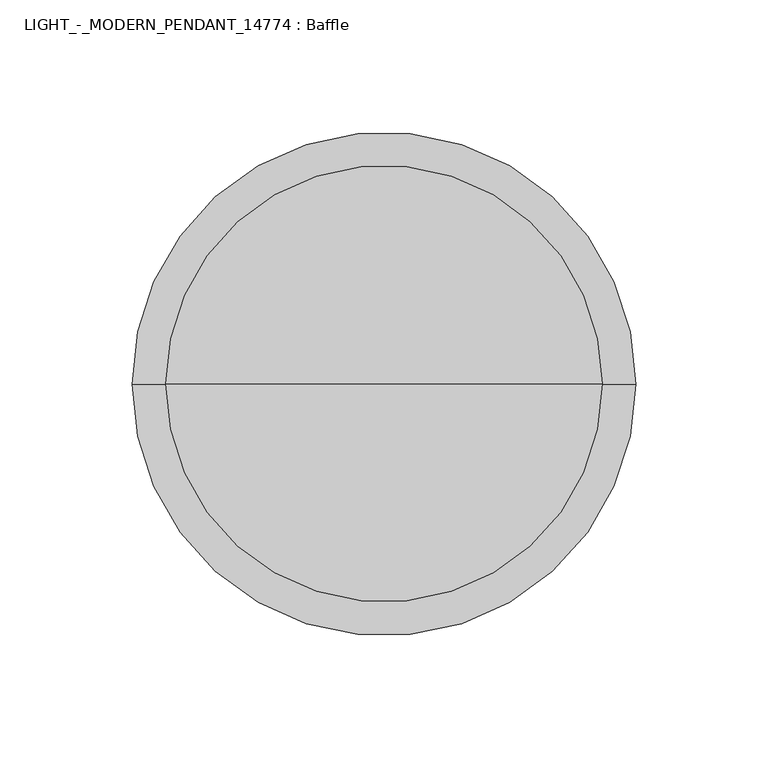
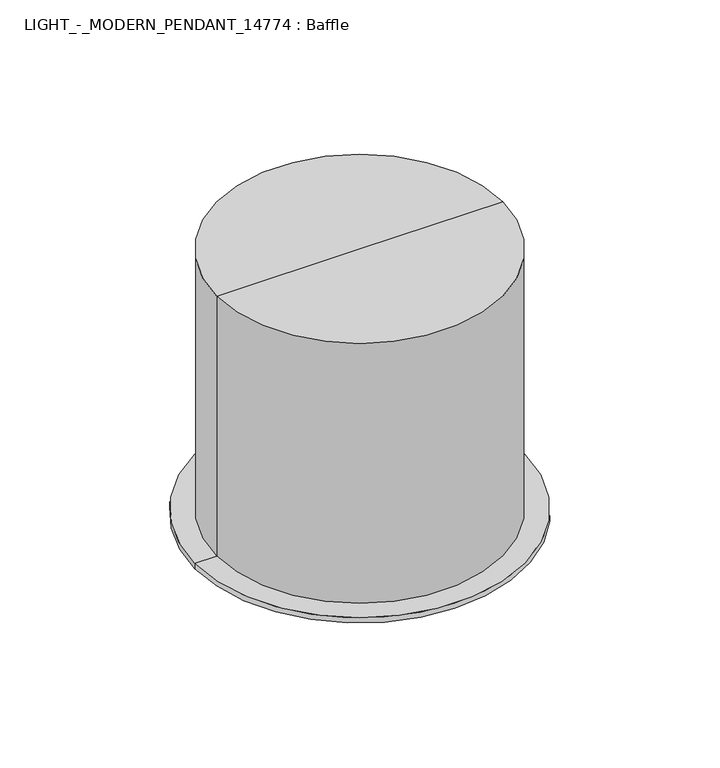
"""IFC4 building model written with IfcOpenShell, lengths in millimetres: light fixture geometry, LIGHT_-_MODERN_PENDANT_14774 : Baffle."""

from ifc_helpers import new_model, si_unit, frame, origin, place, context, project, spatial, polyline, circle_curve, source, transform, mapped, element, save
from ifc_brep_helpers import plane_surface, cylinder_surface, revolved_surface, advanced_brep


def light_modern_pendant_14774_baffle_cc9af11b(model_context):
    return source(origin(), model_context, "Body", "AdvancedBrep", [
        advanced_brep(
        [(-76.2, 0.0, 2438.4), (76.2, 0.0, 2438.4), (76.2, 0.0, 2590.8), (-76.2, 0.0, 2590.8), (-82.55, 0.0, 2438.4), (82.55, 0.0, 2438.4), (-82.55, 0.0, 2597.15), (82.55, 0.0, 2597.15), (0.0, 0.0, 2597.15), (0.0, 0.0, 2590.8)],
        [
            (0, 1, circle_curve(frame((0.0, 0.0, 2438.4), z_axis=(0.0, 0.0, -1.0), x_axis=(1.0, 0.0, 0.0)), 76.2)),
            (1, 2),
            (2, 3, circle_curve(frame((0.0, 0.0, 2590.8), z_axis=(0.0, 0.0, 1.0), x_axis=(1.0, 0.0, 0.0)), 76.2)),
            (3, 0),
            (1, 0, circle_curve(frame((0.0, 0.0, 2438.4), z_axis=(0.0, 0.0, -1.0), x_axis=(1.0, 0.0, 0.0)), 76.2)),
            (3, 2, circle_curve(frame((0.0, 0.0, 2590.8), z_axis=(0.0, 0.0, 1.0), x_axis=(1.0, 0.0, 0.0)), 76.2)),
            (4, 5, circle_curve(frame((0.0, 0.0, 2438.4), z_axis=(0.0, 0.0, -1.0), x_axis=(1.0, 0.0, 0.0)), 82.55)),
            (5, 1),
            (0, 4),
            (5, 4, circle_curve(frame((0.0, 0.0, 2438.4), z_axis=(0.0, 0.0, -1.0), x_axis=(1.0, 0.0, 0.0)), 82.55)),
            (6, 7, circle_curve(frame((0.0, 0.0, 2597.15), z_axis=(0.0, 0.0, -1.0), x_axis=(1.0, 0.0, 0.0)), 82.55)),
            (7, 5),
            (4, 6),
            (7, 6, circle_curve(frame((0.0, 0.0, 2597.15), z_axis=(0.0, 0.0, -1.0), x_axis=(1.0, 0.0, 0.0)), 82.55)),
            (8, 7),
            (6, 8),
            (2, 9),
            (9, 3),
        ],
        [
            revolved_surface(polyline([(76.2, 0.0, 2590.8), (76.2, 0.0, 2438.4)]), (0.0, 0.0, 2438.4), (0.0, 0.0, 1.0)),
            plane_surface(frame((0.0, 0.0, 2438.4), z_axis=(0.0, 0.0, -1.0), x_axis=(1.0, 0.0, 0.0))),
            cylinder_surface(frame((0.0, 0.0, 2438.4), z_axis=(0.0, 0.0, 1.0), x_axis=(1.0, 0.0, 0.0)), 82.55),
            plane_surface(frame((0.0, 0.0, 2597.15), z_axis=(0.0, 0.0, 1.0), x_axis=(1.0, 0.0, 0.0))),
            plane_surface(frame((0.0, 0.0, 2590.8), z_axis=(0.0, 0.0, -1.0), x_axis=(1.0, 0.0, 0.0))),
        ],
        [
            (0, [[1, 2, 3, 4]]),
            (0, [[5, -4, 6, -2]]),
            (1, [[7, 8, -1, 9]]),
            (1, [[10, -9, -5, -8]]),
            (2, [[11, 12, -7, 13]]),
            (2, [[14, -13, -10, -12]]),
            (3, [[15, -11, 16]]),
            (3, [[-16, -14, -15]]),
            (4, [[-3, 17, 18]]),
            (4, [[-6, -18, -17]]),
        ],
    ),
        advanced_brep(
        [(76.2, 0.0, 2473.3352136), (-76.2, 0.0, 2473.3352136), (-66.6647864, 0.0, 2463.8), (66.6647864, 0.0, 2463.8), (76.2, 0.0, 2438.4), (-76.2, 0.0, 2438.4), (71.3980217, 0.0, 2438.4), (-71.3980217, 0.0, 2438.4), (71.3980217, 0.0, 2444.75), (-71.3980217, 0.0, 2444.75), (69.8397864, 0.0, 2444.75), (-69.8397864, 0.0, 2444.75), (69.8397864, 0.0, 2451.1), (-69.8397864, 0.0, 2451.1), (68.2522864, 0.0, 2451.1), (-68.2522864, 0.0, 2451.1), (68.2522864, 0.0, 2457.45), (-68.2522864, 0.0, 2457.45), (66.6647864, 0.0, 2457.45), (-66.6647864, 0.0, 2457.45)],
        [
            (0, 1, circle_curve(frame((0.0, 0.0, 2473.3352136), z_axis=(0.0, 0.0, 1.0), x_axis=(-1.0, 0.0, 0.0)), 76.2)),
            (1, 2),
            (2, 3, circle_curve(frame((0.0, 0.0, 2463.8), z_axis=(0.0, 0.0, -1.0), x_axis=(-1.0, 0.0, 0.0)), 66.6647864)),
            (3, 0),
            (1, 0, circle_curve(frame((0.0, 0.0, 2473.3352136), z_axis=(0.0, 0.0, 1.0), x_axis=(-1.0, 0.0, 0.0)), 76.2)),
            (3, 2, circle_curve(frame((0.0, 0.0, 2463.8), z_axis=(0.0, 0.0, -1.0), x_axis=(-1.0, 0.0, 0.0)), 66.6647864)),
            (4, 5, circle_curve(frame((0.0, 0.0, 2438.4), z_axis=(0.0, 0.0, 1.0), x_axis=(-1.0, 0.0, 0.0)), 76.2)),
            (5, 1),
            (0, 4),
            (5, 4, circle_curve(frame((0.0, 0.0, 2438.4), z_axis=(0.0, 0.0, 1.0), x_axis=(-1.0, 0.0, 0.0)), 76.2)),
            (6, 7, circle_curve(frame((0.0, 0.0, 2438.4), z_axis=(0.0, 0.0, 1.0), x_axis=(-1.0, 0.0, 0.0)), 71.3980217)),
            (7, 5),
            (4, 6),
            (7, 6, circle_curve(frame((0.0, 0.0, 2438.4), z_axis=(0.0, 0.0, 1.0), x_axis=(-1.0, 0.0, 0.0)), 71.3980217)),
            (8, 9, circle_curve(frame((0.0, 0.0, 2444.75), z_axis=(0.0, 0.0, 1.0), x_axis=(-1.0, 0.0, 0.0)), 71.3980217)),
            (9, 7),
            (6, 8),
            (9, 8, circle_curve(frame((0.0, 0.0, 2444.75), z_axis=(0.0, 0.0, 1.0), x_axis=(-1.0, 0.0, 0.0)), 71.3980217)),
            (10, 11, circle_curve(frame((0.0, 0.0, 2444.75), z_axis=(0.0, 0.0, 1.0), x_axis=(-1.0, 0.0, 0.0)), 69.8397864)),
            (11, 9),
            (8, 10),
            (11, 10, circle_curve(frame((0.0, 0.0, 2444.75), z_axis=(0.0, 0.0, 1.0), x_axis=(-1.0, 0.0, 0.0)), 69.8397864)),
            (12, 13, circle_curve(frame((0.0, 0.0, 2451.1), z_axis=(0.0, 0.0, 1.0), x_axis=(-1.0, 0.0, 0.0)), 69.8397864)),
            (13, 11),
            (10, 12),
            (13, 12, circle_curve(frame((0.0, 0.0, 2451.1), z_axis=(0.0, 0.0, 1.0), x_axis=(-1.0, 0.0, 0.0)), 69.8397864)),
            (14, 15, circle_curve(frame((0.0, 0.0, 2451.1), z_axis=(0.0, 0.0, 1.0), x_axis=(-1.0, 0.0, 0.0)), 68.2522864)),
            (15, 13),
            (12, 14),
            (15, 14, circle_curve(frame((0.0, 0.0, 2451.1), z_axis=(0.0, 0.0, 1.0), x_axis=(-1.0, 0.0, 0.0)), 68.2522864)),
            (16, 17, circle_curve(frame((0.0, 0.0, 2457.45), z_axis=(0.0, 0.0, 1.0), x_axis=(-1.0, 0.0, 0.0)), 68.2522864)),
            (17, 15),
            (14, 16),
            (17, 16, circle_curve(frame((0.0, 0.0, 2457.45), z_axis=(0.0, 0.0, 1.0), x_axis=(-1.0, 0.0, 0.0)), 68.2522864)),
            (18, 19, circle_curve(frame((0.0, 0.0, 2457.45), z_axis=(0.0, 0.0, 1.0), x_axis=(-1.0, 0.0, 0.0)), 66.6647864)),
            (19, 17),
            (16, 18),
            (19, 18, circle_curve(frame((0.0, 0.0, 2457.45), z_axis=(0.0, 0.0, 1.0), x_axis=(-1.0, 0.0, 0.0)), 66.6647864)),
            (2, 19),
            (18, 3),
        ],
        [
            revolved_surface(polyline([(-66.6647864, 0.0, 2463.8), (-76.2, 0.0, 2473.3352136)]), (0.0, 0.0, 2584.45), (0.0, 0.0, -1.0)),
            cylinder_surface(frame((0.0, 0.0, 2584.45), z_axis=(0.0, 0.0, -1.0), x_axis=(-1.0, 0.0, 0.0)), 76.2),
            plane_surface(frame((0.0, 0.0, 2438.4), z_axis=(0.0, 0.0, -1.0), x_axis=(-1.0, 0.0, 0.0))),
            revolved_surface(polyline([(-71.3980217, 0.0, 2438.4), (-71.3980217, 0.0, 2444.75)]), (0.0, 0.0, 2584.45), (0.0, 0.0, -1.0)),
            plane_surface(frame((0.0, 0.0, 2444.75), z_axis=(0.0, 0.0, -1.0), x_axis=(-1.0, 0.0, 0.0))),
            revolved_surface(polyline([(-69.8397864, 0.0, 2444.75), (-69.8397864, 0.0, 2451.1)]), (0.0, 0.0, 2584.45), (0.0, 0.0, -1.0)),
            plane_surface(frame((0.0, 0.0, 2451.1), z_axis=(0.0, 0.0, -1.0), x_axis=(-1.0, 0.0, 0.0))),
            revolved_surface(polyline([(-68.2522864, 0.0, 2451.1), (-68.2522864, 0.0, 2457.45)]), (0.0, 0.0, 2584.45), (0.0, 0.0, -1.0)),
            plane_surface(frame((0.0, 0.0, 2457.45), z_axis=(0.0, 0.0, -1.0), x_axis=(-1.0, 0.0, 0.0))),
            revolved_surface(polyline([(-66.6647864, 0.0, 2457.45), (-66.6647864, 0.0, 2463.8)]), (0.0, 0.0, 2584.45), (0.0, 0.0, -1.0)),
        ],
        [
            (0, [[1, 2, 3, 4]]),
            (0, [[5, -4, 6, -2]]),
            (1, [[7, 8, -1, 9]]),
            (1, [[10, -9, -5, -8]]),
            (2, [[11, 12, -7, 13]]),
            (2, [[14, -13, -10, -12]]),
            (3, [[15, 16, -11, 17]]),
            (3, [[18, -17, -14, -16]]),
            (4, [[19, 20, -15, 21]]),
            (4, [[22, -21, -18, -20]]),
            (5, [[23, 24, -19, 25]]),
            (5, [[26, -25, -22, -24]]),
            (6, [[27, 28, -23, 29]]),
            (6, [[30, -29, -26, -28]]),
            (7, [[31, 32, -27, 33]]),
            (7, [[34, -33, -30, -32]]),
            (8, [[35, 36, -31, 37]]),
            (8, [[38, -37, -34, -36]]),
            (9, [[-3, 39, -35, 40]]),
            (9, [[-6, -40, -38, -39]]),
        ],
    ),
        advanced_brep(
        [(73.0147864, 0.0, 2438.4), (-73.0147864, 0.0, 2438.4), (-73.0147864, 0.0, 2432.05), (73.0147864, 0.0, 2432.05), (95.25, 0.0, 2438.4), (-95.25, 0.0, 2438.4), (95.25, 0.0, 2435.1749555), (-95.25, 0.0, 2435.1749555), (76.2, 0.0, 2432.05), (-76.2, 0.0, 2432.05)],
        [
            (0, 1, circle_curve(frame((0.0, 0.0, 2438.4), z_axis=(0.0, 0.0, 1.0), x_axis=(-1.0, 0.0, 0.0)), 73.0147864)),
            (1, 2),
            (2, 3, circle_curve(frame((0.0, 0.0, 2432.05), z_axis=(0.0, 0.0, -1.0), x_axis=(-1.0, 0.0, 0.0)), 73.0147864)),
            (3, 0),
            (1, 0, circle_curve(frame((0.0, 0.0, 2438.4), z_axis=(0.0, 0.0, 1.0), x_axis=(-1.0, 0.0, 0.0)), 73.0147864)),
            (3, 2, circle_curve(frame((0.0, 0.0, 2432.05), z_axis=(0.0, 0.0, -1.0), x_axis=(-1.0, 0.0, 0.0)), 73.0147864)),
            (4, 5, circle_curve(frame((0.0, 0.0, 2438.4), z_axis=(0.0, 0.0, 1.0), x_axis=(-1.0, 0.0, 0.0)), 95.25)),
            (5, 1),
            (0, 4),
            (5, 4, circle_curve(frame((0.0, 0.0, 2438.4), z_axis=(0.0, 0.0, 1.0), x_axis=(-1.0, 0.0, 0.0)), 95.25)),
            (6, 7, circle_curve(frame((0.0, 0.0, 2435.1749555), z_axis=(0.0, 0.0, 1.0), x_axis=(-1.0, 0.0, 0.0)), 95.25)),
            (7, 5),
            (4, 6),
            (7, 6, circle_curve(frame((0.0, 0.0, 2435.1749555), z_axis=(0.0, 0.0, 1.0), x_axis=(-1.0, 0.0, 0.0)), 95.25)),
            (8, 9, circle_curve(frame((0.0, 0.0, 2432.05), z_axis=(0.0, 0.0, 1.0), x_axis=(-1.0, 0.0, 0.0)), 76.2)),
            (9, 7),
            (6, 8),
            (9, 8, circle_curve(frame((0.0, 0.0, 2432.05), z_axis=(0.0, 0.0, 1.0), x_axis=(-1.0, 0.0, 0.0)), 76.2)),
            (2, 9),
            (8, 3),
        ],
        [
            revolved_surface(polyline([(-73.0147864, 0.0, 2432.05), (-73.0147864, 0.0, 2438.4)]), (0.0, 0.0, 2584.45), (0.0, 0.0, -1.0)),
            plane_surface(frame((0.0, 0.0, 2438.4), z_axis=(0.0, 0.0, 1.0), x_axis=(-1.0, 0.0, 0.0))),
            cylinder_surface(frame((0.0, 0.0, 2584.45), z_axis=(0.0, 0.0, -1.0), x_axis=(-1.0, 0.0, 0.0)), 95.25),
            revolved_surface(polyline([(-95.25, 0.0, 2435.1749555), (-76.2, 0.0, 2432.05)]), (0.0, 0.0, 2584.45), (0.0, 0.0, -1.0)),
            plane_surface(frame((0.0, 0.0, 2432.05), z_axis=(0.0, 0.0, -1.0), x_axis=(-1.0, 0.0, 0.0))),
        ],
        [
            (0, [[1, 2, 3, 4]]),
            (0, [[5, -4, 6, -2]]),
            (1, [[7, 8, -1, 9]]),
            (1, [[10, -9, -5, -8]]),
            (2, [[11, 12, -7, 13]]),
            (2, [[14, -13, -10, -12]]),
            (3, [[15, 16, -11, 17]]),
            (3, [[18, -17, -14, -16]]),
            (4, [[-3, 19, -15, 20]]),
            (4, [[-6, -20, -18, -19]]),
        ],
    ),
    ])


if __name__ == "__main__":
    model = new_model("IFC4")
    model_context = context("Model", 3, world=origin())
    ifc_project = project(units=[si_unit("LENGTHUNIT", "METRE", prefix="MILLI")], contexts=[model_context])
    site = spatial("IfcSite", under=ifc_project)
    building = spatial("IfcBuilding", under=site)
    placement = place(None, origin())
    light_modern_pendant_14774_baffle_shape = light_modern_pendant_14774_baffle_cc9af11b(model_context)
    element("IfcLightFixture", 1, ObjectType="LIGHT_-_MODERN_PENDANT_14774 : Baffle", at=placement, inside=building, context=model_context, shape_type="MappedRepresentation", body=[
        mapped(light_modern_pendant_14774_baffle_shape, transform((0.0, 0.0, 0.0), x_axis=(1.0, 0.0, 0.0), y_axis=(0.0, 1.0, 0.0), z_axis=(0.0, 0.0, 1.0))),
    ])
    save(model, "model.ifc")

# Revit data of these elements
# Type "LIGHT_-_MODERN_PENDANT_14774 : Baffle"
#   Assembly Code = "D5020220"
#   Lamp = "A-19"
#   Wattage Comments = "60"
#   Wattage = 7.27067 W
#   built-in parameter 1150110 = 1 (stored number, unit not read)
#   built-in parameter 1114217 = 1 (stored number, unit not read)
#   Tilt Angle = 60.00°
#   built-in parameter 1150109 = 1 (stored number, unit not read)
#   built-in parameter 1150113 = 1 (stored number, unit not read)
#   built-in parameter 1010507 = 1.5708 (stored number, unit not read)
#   built-in parameter 1010506 = 0.523599 (stored number, unit not read)
#   built-in parameter 1150105 = 3611.05 (stored number, unit not read)
#   built-in parameter 1150115 = 1 (stored number, unit not read)
#   Light Source Symbol Length = 10' - 0"
#   built-in parameter 1150112 = 1 (stored number, unit not read)
#   built-in parameter 1150114 = 1 (stored number, unit not read)
#   built-in parameter 1150107 = 3200 (stored number, unit not read)
#   built-in parameter 1150106 = 36.1105 (stored number, unit not read)
#   built-in parameter 1150104 = 13.8 (stored number, unit not read)
#   built-in parameter 1114218 = 1 (stored number, unit not read)
#   built-in parameter 1150133 = 10 (stored number, unit not read)
#   Depth = 0' - 8"
#   Diameter = 0' - 6"
#   Lumens = 1080 lm
#   Wall Washer = no
#   Wall Wash Trim = no
#   built-in parameter 1150134 = 3
#   Reflector Cone = no
#   built-in parameter 1150132 = 2
#   Fresnel Lens = no
#   Color Filter = 16777215
#   Baffle = yes
#   Wall Wash Reflector [instance default] = none
#   Reflector [instance default] = none
#   Light Trim = Metal - Paint Finish - Ivory,Glossy
#   Fresnel Material [instance default] = none
#   Dimming Lamp Color Temperature Shift = (empty or 0)
#   Default Elevation = 0
# Element 1 (IfcLightFixture, "LIGHT_-_MODERN_PENDANT_14774 : Baffle")
#   Materials on its faces: "Metal - Paint Finish - Ivory,Glossy"
# Materials
#   "Metal - Paint Finish - Ivory,Glossy": colour RGB 247 247 239, transparency 0
